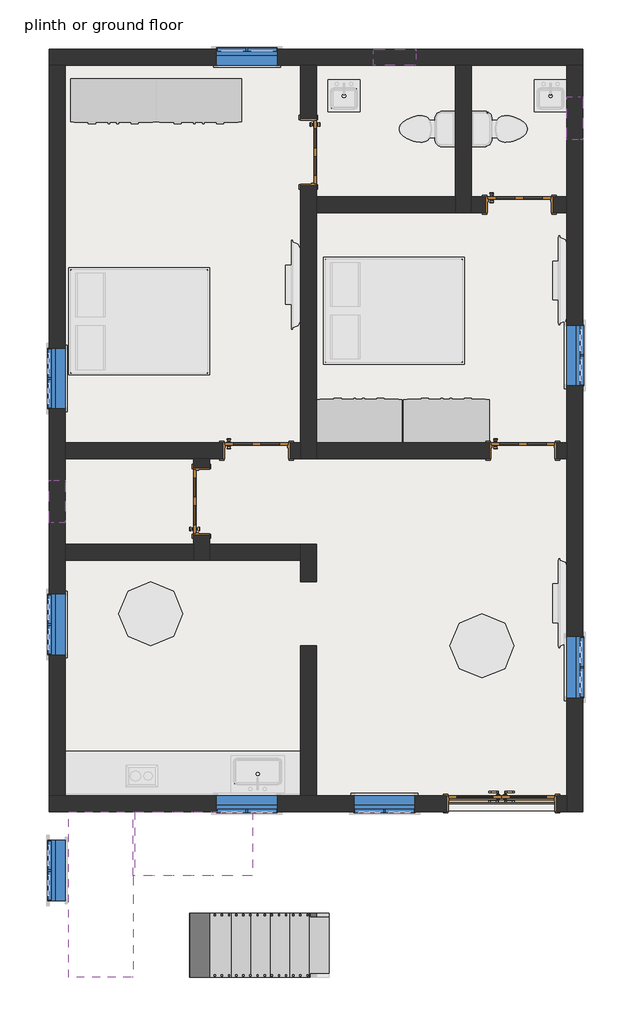
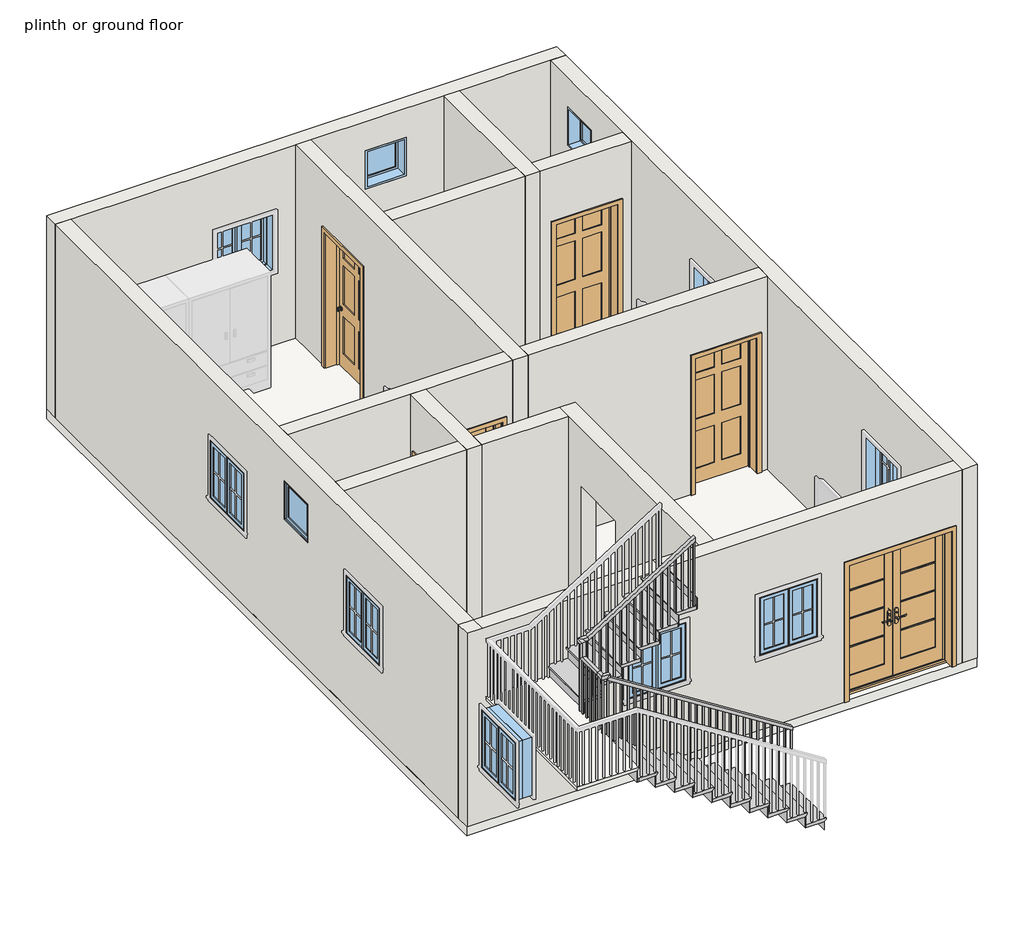
# One storey, part 1 of 3: 14 walls, 11 windows, 6 doors, 2 slabs, 2 stair flights, 1 railing.
"""IFC4 building model written with IfcOpenShell, lengths in millimetres."""

from ifc_helpers import new_model, si_unit, frame, origin, place, context, project, spatial, polyline, outline, extrude, faceted_brep, transform, mapped, element, save
from components import door_7ffae4ec, door_d86b6c54, non_monolithic_landing_b7697d37, stair_flight_c6e2231d, stair_flight_b29bf434, window_80340324, window_339605e1

model = new_model("IFC4")

# Units and contexts
model_context = context("Model", 3, world=origin())
ifc_project = project(units=[si_unit("LENGTHUNIT", "METRE", prefix="MILLI")], contexts=[model_context])

# Site, building, storey
site = spatial("IfcSite", under=ifc_project)
building = spatial("IfcBuilding", under=site)
storey = spatial("IfcBuildingStorey", under=building, Name="plinth or ground floor", Elevation=609.6)

# Doors
placement = place(None, origin())
door_shape = door_7ffae4ec(model_context)
element("IfcDoor", 1, ObjectType="Door-Exterior-Double-Full Glass-Wood_Clad : 60\" x 84\"", at=placement, inside=storey, context=model_context, shape_type="MappedRepresentation", body=[
    mapped(door_shape, transform((25464.9136801, 6450.5159313, 609.6), x_axis=(1.0, 0.0, 0.0), y_axis=(0.0, 1.0, 0.0), z_axis=(0.0, 0.0, 1.0))),
])
door_2_shape = door_d86b6c54(model_context)
element("IfcDoor", 2, ObjectType="Door-Interior-Single-6_Panel-Wood : 36\" x 84\"", at=placement, inside=storey, context=model_context, shape_type="MappedRepresentation", body=[
    mapped(door_2_shape, transform((25769.7136801, 11479.7159313, 609.6), x_axis=(1.0, 0.0, 0.0), y_axis=(0.0, 1.0, 0.0), z_axis=(0.0, 0.0, 1.0))),
])
element("IfcDoor", 3, ObjectType="Door-Interior-Single-6_Panel-Wood : 36\" x 84\"", at=placement, inside=storey, context=model_context, shape_type="MappedRepresentation", body=[
    mapped(door_2_shape, transform((21969.5484036, 11479.7159313, 609.6), x_axis=(1.0, 0.0, 0.0), y_axis=(0.0, 1.0, 0.0), z_axis=(0.0, 0.0, 1.0))),
])
element("IfcDoor", 4, ObjectType="Door-Interior-Single-6_Panel-Wood : 36\" x 84\"", at=placement, inside=storey, context=model_context, shape_type="MappedRepresentation", body=[
    mapped(door_2_shape, transform((22712.1886801, 15731.0409313, 609.6), x_axis=(0.0, -1.0, 0.0), y_axis=(1.0, 0.0, 0.0), z_axis=(0.0, 0.0, 1.0))),
])
element("IfcDoor", 5, ObjectType="Door-Interior-Single-6_Panel-Wood : 36\" x 84\"", at=placement, inside=storey, context=model_context, shape_type="MappedRepresentation", body=[
    mapped(door_2_shape, transform((25718.9136801, 14984.9159313, 609.6), x_axis=(1.0, 0.0, 0.0), y_axis=(0.0, 1.0, 0.0), z_axis=(0.0, 0.0, 1.0))),
])
element("IfcDoor", 6, ObjectType="Door-Interior-Single-6_Panel-Wood : 36\" x 84\"", at=placement, inside=storey, context=model_context, shape_type="MappedRepresentation", body=[
    mapped(door_2_shape, transform((21181.8386801, 10752.6409313, 609.6), x_axis=(0.0, 1.0, 0.0), y_axis=(-1.0, 0.0, 0.0), z_axis=(0.0, 0.0, 1.0))),
])

# Railing
element("IfcRailing", 7, ObjectType="Handrail - Rectangular", at=placement, inside=storey, context=model_context, shape_type="SolidModel", body=[
    faceted_brep([(23001.1136801, 4834.4409313, 1701.8), (23001.1136801, 4834.4409313, 1641.586276), (23001.1136801, 4885.2409313, 1641.586276), (23001.1136801, 4885.2409313, 1701.8), (20283.3136801, 4834.4409313, 3431.3090909), (20232.5136801, 4834.4409313, 3403.4226396), (20232.5136801, 4885.2409313, 3403.4226396), (20283.3136801, 4885.2409313, 3431.3090909), (20283.3136801, 4834.4409313, 3479.8), (20232.5136801, 4834.4409313, 3429.0), (20232.5136801, 4885.2409313, 3429.0), (20283.3136801, 4885.2409313, 3479.8), (20156.3136801, 4834.4409313, 3479.8), (20156.3136801, 4834.4409313, 3429.0), (20207.1136801, 4885.2409313, 3429.0), (20207.1136801, 4885.2409313, 3479.8), (20156.3136801, 4961.4409313, 3479.8), (20156.3136801, 4961.4409313, 3429.0), (20207.1136801, 4961.4409313, 3429.0), (20207.1136801, 4961.4409313, 3479.8), (20156.3136801, 5342.4409313, 3479.8), (20156.3136801, 5393.2409313, 3429.0), (20207.1136801, 5393.2409313, 3429.0), (20207.1136801, 5342.4409313, 3479.8), (20156.3136801, 5342.4409313, 3706.0909091), (20156.3136801, 5393.2409313, 3655.2909091), (20207.1136801, 5393.2409313, 3655.2909091), (20207.1136801, 5342.4409313, 3706.0909091), (20156.3136801, 5469.4409313, 3706.0909091), (20156.3136801, 5469.4409313, 3655.2909091), (20207.1136801, 5418.6409313, 3655.2909091), (20207.1136801, 5418.6409313, 3706.0909091), (20283.3136801, 5469.4409313, 3706.0909091), (20298.106675, 5469.4409313, 3655.2909091), (20298.106675, 5418.6409313, 3655.2909091), (20283.3136801, 5418.6409313, 3706.0909091), (21883.5136801, 5469.4409313, 4724.4), (21883.5136801, 5418.6409313, 4724.4), (21883.5136801, 5418.6409313, 4664.186276), (21883.5136801, 5469.4409313, 4664.186276)], [[[0, 1, 2, 3]], [[1, 0, 4, 5]], [[2, 1, 5, 6]], [[3, 2, 6, 7]], [[0, 3, 7, 4]], [[5, 4, 8, 9]], [[6, 5, 9, 10]], [[7, 6, 10, 11]], [[4, 7, 11, 8]], [[9, 8, 12, 13]], [[10, 9, 13, 14]], [[11, 10, 14, 15]], [[8, 11, 15, 12]], [[13, 12, 16, 17]], [[14, 13, 17, 18]], [[15, 14, 18, 19]], [[12, 15, 19, 16]], [[17, 16, 20, 21]], [[18, 17, 21, 22]], [[19, 18, 22, 23]], [[16, 19, 23, 20]], [[21, 20, 24, 25]], [[22, 21, 25, 26]], [[23, 22, 26, 27]], [[20, 23, 27, 24]], [[25, 24, 28, 29]], [[26, 25, 29, 30]], [[27, 26, 30, 31]], [[24, 27, 31, 28]], [[29, 28, 32, 33]], [[30, 29, 33, 34]], [[31, 30, 34, 35]], [[28, 31, 35, 32]], [[36, 37, 38, 39]], [[33, 32, 36, 39]], [[34, 33, 39, 38]], [[35, 34, 38, 37]], [[32, 35, 37, 36]]]),
    extrude(outline(polyline([(4621.7567305, 21816.8386801), (4609.6340032, 21797.7886801), (3632.2, 21797.7886801), (3632.2, 21816.8386801), (4621.7567305, 21816.8386801)])), frame((0.0, 5434.5159313, 0.0), z_axis=(0.0, 1.0, 0.0), x_axis=(0.0, 0.0, 1.0)), (0.0, 0.0, 1.0), 19.05),
    extrude(outline(polyline([(4557.1021851, 21715.2386801), (4544.9794578, 21696.1886801), (3632.2, 21696.1886801), (3632.2, 21715.2386801), (4557.1021851, 21715.2386801)])), frame((0.0, 5434.5159313, 0.0), z_axis=(0.0, 1.0, 0.0), x_axis=(0.0, 0.0, 1.0)), (0.0, 0.0, 1.0), 19.05),
    extrude(outline(polyline([(4492.4476396, 21613.6386801), (4480.3249123, 21594.5886801), (3632.2, 21594.5886801), (3632.2, 21613.6386801), (4492.4476396, 21613.6386801)])), frame((0.0, 5434.5159313, 0.0), z_axis=(0.0, 1.0, 0.0), x_axis=(0.0, 0.0, 1.0)), (0.0, 0.0, 1.0), 19.05),
    extrude(outline(polyline([(4427.7930941, 21512.0386801), (4415.6703669, 21492.9886801), (3454.4, 21492.9886801), (3454.4, 21512.0386801), (4427.7930941, 21512.0386801)])), frame((0.0, 5434.5159313, 0.0), z_axis=(0.0, 1.0, 0.0), x_axis=(0.0, 0.0, 1.0)), (0.0, 0.0, 1.0), 19.05),
    extrude(outline(polyline([(4363.1385487, 21410.4386801), (4351.0158214, 21391.3886801), (3454.4, 21391.3886801), (3454.4, 21410.4386801), (4363.1385487, 21410.4386801)])), frame((0.0, 5434.5159313, 0.0), z_axis=(0.0, 1.0, 0.0), x_axis=(0.0, 0.0, 1.0)), (0.0, 0.0, 1.0), 19.05),
    extrude(outline(polyline([(4298.4840032, 21308.8386801), (4286.361276, 21289.7886801), (3276.6, 21289.7886801), (3276.6, 21308.8386801), (4298.4840032, 21308.8386801)])), frame((0.0, 5434.5159313, 0.0), z_axis=(0.0, 1.0, 0.0), x_axis=(0.0, 0.0, 1.0)), (0.0, 0.0, 1.0), 19.05),
    extrude(outline(polyline([(4233.8294578, 21207.2386801), (4221.7067305, 21188.1886801), (3276.6, 21188.1886801), (3276.6, 21207.2386801), (4233.8294578, 21207.2386801)])), frame((0.0, 5434.5159313, 0.0), z_axis=(0.0, 1.0, 0.0), x_axis=(0.0, 0.0, 1.0)), (0.0, 0.0, 1.0), 19.05),
    extrude(outline(polyline([(4169.1749123, 21105.6386801), (4157.0521851, 21086.5886801), (3276.6, 21086.5886801), (3276.6, 21105.6386801), (4169.1749123, 21105.6386801)])), frame((0.0, 5434.5159313, 0.0), z_axis=(0.0, 1.0, 0.0), x_axis=(0.0, 0.0, 1.0)), (0.0, 0.0, 1.0), 19.05),
    extrude(outline(polyline([(4104.5203669, 21004.0386801), (4092.3976396, 20984.9886801), (3098.8, 20984.9886801), (3098.8, 21004.0386801), (4104.5203669, 21004.0386801)])), frame((0.0, 5434.5159313, 0.0), z_axis=(0.0, 1.0, 0.0), x_axis=(0.0, 0.0, 1.0)), (0.0, 0.0, 1.0), 19.05),
    extrude(outline(polyline([(4039.8658214, 20902.4386801), (4027.7430941, 20883.3886801), (3098.8, 20883.3886801), (3098.8, 20902.4386801), (4039.8658214, 20902.4386801)])), frame((0.0, 5434.5159313, 0.0), z_axis=(0.0, 1.0, 0.0), x_axis=(0.0, 0.0, 1.0)), (0.0, 0.0, 1.0), 19.05),
    extrude(outline(polyline([(3975.211276, 20800.8386801), (3963.0885487, 20781.7886801), (3098.8, 20781.7886801), (3098.8, 20800.8386801), (3975.211276, 20800.8386801)])), frame((0.0, 5434.5159313, 0.0), z_axis=(0.0, 1.0, 0.0), x_axis=(0.0, 0.0, 1.0)), (0.0, 0.0, 1.0), 19.05),
    extrude(outline(polyline([(3910.5567305, 20699.2386801), (3898.4340032, 20680.1886801), (2921.0, 20680.1886801), (2921.0, 20699.2386801), (3910.5567305, 20699.2386801)])), frame((0.0, 5434.5159313, 0.0), z_axis=(0.0, 1.0, 0.0), x_axis=(0.0, 0.0, 1.0)), (0.0, 0.0, 1.0), 19.05),
    extrude(outline(polyline([(3845.9021851, 20597.6386801), (3833.7794578, 20578.5886801), (2921.0, 20578.5886801), (2921.0, 20597.6386801), (3845.9021851, 20597.6386801)])), frame((0.0, 5434.5159313, 0.0), z_axis=(0.0, 1.0, 0.0), x_axis=(0.0, 0.0, 1.0)), (0.0, 0.0, 1.0), 19.05),
    extrude(outline(polyline([(3781.2476396, 20496.0386801), (3769.1249123, 20476.9886801), (2921.0, 20476.9886801), (2921.0, 20496.0386801), (3781.2476396, 20496.0386801)])), frame((0.0, 5434.5159313, 0.0), z_axis=(0.0, 1.0, 0.0), x_axis=(0.0, 0.0, 1.0)), (0.0, 0.0, 1.0), 19.05),
    extrude(outline(polyline([(3716.5930941, 20394.4386801), (3704.4703669, 20375.3886801), (2743.2, 20375.3886801), (2743.2, 20394.4386801), (3716.5930941, 20394.4386801)])), frame((0.0, 5434.5159313, 0.0), z_axis=(0.0, 1.0, 0.0), x_axis=(0.0, 0.0, 1.0)), (0.0, 0.0, 1.0), 19.05),
    extrude(outline(polyline([(3651.9385487, 20292.8386801), (3639.8158214, 20273.7886801), (2743.2, 20273.7886801), (2743.2, 20292.8386801), (3651.9385487, 20292.8386801)])), frame((0.0, 5434.5159313, 0.0), z_axis=(0.0, 1.0, 0.0), x_axis=(0.0, 0.0, 1.0)), (0.0, 0.0, 1.0), 19.05),
    extrude(outline(polyline([(20191.2386801, 5358.3159313), (20172.1886801, 5358.3159313), (20172.1886801, 5377.3659313), (20191.2386801, 5377.3659313), (20191.2386801, 5358.3159313)])), frame((0.0, 0.0, 2565.4), z_axis=(0.0, 0.0, 1.0), x_axis=(1.0, 0.0, 0.0)), (0.0, 0.0, 1.0), 1089.8909091),
    extrude(outline(polyline([(20191.2386801, 5256.7159313), (20172.1886801, 5256.7159313), (20172.1886801, 5275.7659313), (20191.2386801, 5275.7659313), (20191.2386801, 5256.7159313)])), frame((0.0, 0.0, 2565.4), z_axis=(0.0, 0.0, 1.0), x_axis=(1.0, 0.0, 0.0)), (0.0, 0.0, 1.0), 863.6),
    extrude(outline(polyline([(20191.2386801, 5155.1159313), (20172.1886801, 5155.1159313), (20172.1886801, 5174.1659313), (20191.2386801, 5174.1659313), (20191.2386801, 5155.1159313)])), frame((0.0, 0.0, 2565.4), z_axis=(0.0, 0.0, 1.0), x_axis=(1.0, 0.0, 0.0)), (0.0, 0.0, 1.0), 863.6),
    extrude(outline(polyline([(20191.2386801, 5053.5159313), (20172.1886801, 5053.5159313), (20172.1886801, 5072.5659313), (20191.2386801, 5072.5659313), (20191.2386801, 5053.5159313)])), frame((0.0, 0.0, 2565.4), z_axis=(0.0, 0.0, 1.0), x_axis=(1.0, 0.0, 0.0)), (0.0, 0.0, 1.0), 863.6),
    extrude(outline(polyline([(20191.2386801, 4951.9159313), (20172.1886801, 4951.9159313), (20172.1886801, 4970.9659313), (20191.2386801, 4970.9659313), (20191.2386801, 4951.9159313)])), frame((0.0, 0.0, 2565.4), z_axis=(0.0, 0.0, 1.0), x_axis=(1.0, 0.0, 0.0)), (0.0, 0.0, 1.0), 863.6),
    extrude(outline(polyline([(20267.4386801, 4869.3659313), (20267.4386801, 4850.3159313), (20248.3886801, 4850.3159313), (20248.3886801, 4869.3659313), (20267.4386801, 4869.3659313)])), frame((0.0, 0.0, 2387.6), z_axis=(0.0, 0.0, 1.0), x_axis=(1.0, 0.0, 0.0)), (0.0, 0.0, 1.0), 1041.4),
    extrude(outline(polyline([(3316.5430941, 20369.0386801), (3328.6658214, 20349.9886801), (2387.6, 20349.9886801), (2387.6, 20369.0386801), (3316.5430941, 20369.0386801)])), frame((0.0, 4850.3159313, 0.0), z_axis=(0.0, 1.0, 0.0), x_axis=(0.0, 0.0, 1.0)), (0.0, 0.0, 1.0), 19.05),
    extrude(outline(polyline([(3251.8885487, 20470.6386801), (3264.011276, 20451.5886801), (2387.6, 20451.5886801), (2387.6, 20470.6386801), (3251.8885487, 20470.6386801)])), frame((0.0, 4850.3159313, 0.0), z_axis=(0.0, 1.0, 0.0), x_axis=(0.0, 0.0, 1.0)), (0.0, 0.0, 1.0), 19.05),
    extrude(outline(polyline([(3187.2340032, 20572.2386801), (3199.3567305, 20553.1886801), (2209.8, 20553.1886801), (2209.8, 20572.2386801), (3187.2340032, 20572.2386801)])), frame((0.0, 4850.3159313, 0.0), z_axis=(0.0, 1.0, 0.0), x_axis=(0.0, 0.0, 1.0)), (0.0, 0.0, 1.0), 19.05),
    extrude(outline(polyline([(3122.5794578, 20673.8386801), (3134.7021851, 20654.7886801), (2209.8, 20654.7886801), (2209.8, 20673.8386801), (3122.5794578, 20673.8386801)])), frame((0.0, 4850.3159313, 0.0), z_axis=(0.0, 1.0, 0.0), x_axis=(0.0, 0.0, 1.0)), (0.0, 0.0, 1.0), 19.05),
    extrude(outline(polyline([(3057.9249123, 20775.4386801), (3070.0476396, 20756.3886801), (2209.8, 20756.3886801), (2209.8, 20775.4386801), (3057.9249123, 20775.4386801)])), frame((0.0, 4850.3159313, 0.0), z_axis=(0.0, 1.0, 0.0), x_axis=(0.0, 0.0, 1.0)), (0.0, 0.0, 1.0), 19.05),
    extrude(outline(polyline([(2993.2703669, 20877.0386801), (3005.3930941, 20857.9886801), (2032.0, 20857.9886801), (2032.0, 20877.0386801), (2993.2703669, 20877.0386801)])), frame((0.0, 4850.3159313, 0.0), z_axis=(0.0, 1.0, 0.0), x_axis=(0.0, 0.0, 1.0)), (0.0, 0.0, 1.0), 19.05),
    extrude(outline(polyline([(2928.6158214, 20978.6386801), (2940.7385487, 20959.5886801), (2032.0, 20959.5886801), (2032.0, 20978.6386801), (2928.6158214, 20978.6386801)])), frame((0.0, 4850.3159313, 0.0), z_axis=(0.0, 1.0, 0.0), x_axis=(0.0, 0.0, 1.0)), (0.0, 0.0, 1.0), 19.05),
    extrude(outline(polyline([(2863.961276, 21080.2386801), (2876.0840032, 21061.1886801), (1854.2, 21061.1886801), (1854.2, 21080.2386801), (2863.961276, 21080.2386801)])), frame((0.0, 4850.3159313, 0.0), z_axis=(0.0, 1.0, 0.0), x_axis=(0.0, 0.0, 1.0)), (0.0, 0.0, 1.0), 19.05),
    extrude(outline(polyline([(2799.3067305, 21181.8386801), (2811.4294578, 21162.7886801), (1854.2, 21162.7886801), (1854.2, 21181.8386801), (2799.3067305, 21181.8386801)])), frame((0.0, 4850.3159313, 0.0), z_axis=(0.0, 1.0, 0.0), x_axis=(0.0, 0.0, 1.0)), (0.0, 0.0, 1.0), 19.05),
    extrude(outline(polyline([(2734.6521851, 21283.4386801), (2746.7749123, 21264.3886801), (1854.2, 21264.3886801), (1854.2, 21283.4386801), (2734.6521851, 21283.4386801)])), frame((0.0, 4850.3159313, 0.0), z_axis=(0.0, 1.0, 0.0), x_axis=(0.0, 0.0, 1.0)), (0.0, 0.0, 1.0), 19.05),
    extrude(outline(polyline([(2669.9976396, 21385.0386801), (2682.1203669, 21365.9886801), (1676.4, 21365.9886801), (1676.4, 21385.0386801), (2669.9976396, 21385.0386801)])), frame((0.0, 4850.3159313, 0.0), z_axis=(0.0, 1.0, 0.0), x_axis=(0.0, 0.0, 1.0)), (0.0, 0.0, 1.0), 19.05),
    extrude(outline(polyline([(2605.3430941, 21486.6386801), (2617.4658214, 21467.5886801), (1676.4, 21467.5886801), (1676.4, 21486.6386801), (2605.3430941, 21486.6386801)])), frame((0.0, 4850.3159313, 0.0), z_axis=(0.0, 1.0, 0.0), x_axis=(0.0, 0.0, 1.0)), (0.0, 0.0, 1.0), 19.05),
    extrude(outline(polyline([(2540.6885487, 21588.2386801), (2552.811276, 21569.1886801), (1676.4, 21569.1886801), (1676.4, 21588.2386801), (2540.6885487, 21588.2386801)])), frame((0.0, 4850.3159313, 0.0), z_axis=(0.0, 1.0, 0.0), x_axis=(0.0, 0.0, 1.0)), (0.0, 0.0, 1.0), 19.05),
    extrude(outline(polyline([(2476.0340032, 21689.8386801), (2488.1567305, 21670.7886801), (1498.6, 21670.7886801), (1498.6, 21689.8386801), (2476.0340032, 21689.8386801)])), frame((0.0, 4850.3159313, 0.0), z_axis=(0.0, 1.0, 0.0), x_axis=(0.0, 0.0, 1.0)), (0.0, 0.0, 1.0), 19.05),
    extrude(outline(polyline([(2411.3794578, 21791.4386801), (2423.5021851, 21772.3886801), (1498.6, 21772.3886801), (1498.6, 21791.4386801), (2411.3794578, 21791.4386801)])), frame((0.0, 4850.3159313, 0.0), z_axis=(0.0, 1.0, 0.0), x_axis=(0.0, 0.0, 1.0)), (0.0, 0.0, 1.0), 19.05),
    extrude(outline(polyline([(2346.7249123, 21893.0386801), (2358.8476396, 21873.9886801), (1498.6, 21873.9886801), (1498.6, 21893.0386801), (2346.7249123, 21893.0386801)])), frame((0.0, 4850.3159313, 0.0), z_axis=(0.0, 1.0, 0.0), x_axis=(0.0, 0.0, 1.0)), (0.0, 0.0, 1.0), 19.05),
    extrude(outline(polyline([(2282.0703669, 21994.6386801), (2294.1930941, 21975.5886801), (1320.8, 21975.5886801), (1320.8, 21994.6386801), (2282.0703669, 21994.6386801)])), frame((0.0, 4850.3159313, 0.0), z_axis=(0.0, 1.0, 0.0), x_axis=(0.0, 0.0, 1.0)), (0.0, 0.0, 1.0), 19.05),
    extrude(outline(polyline([(2217.4158214, 22096.2386801), (2229.5385487, 22077.1886801), (1320.8, 22077.1886801), (1320.8, 22096.2386801), (2217.4158214, 22096.2386801)])), frame((0.0, 4850.3159313, 0.0), z_axis=(0.0, 1.0, 0.0), x_axis=(0.0, 0.0, 1.0)), (0.0, 0.0, 1.0), 19.05),
    extrude(outline(polyline([(2152.761276, 22197.8386801), (2164.8840032, 22178.7886801), (1143.0, 22178.7886801), (1143.0, 22197.8386801), (2152.761276, 22197.8386801)])), frame((0.0, 4850.3159313, 0.0), z_axis=(0.0, 1.0, 0.0), x_axis=(0.0, 0.0, 1.0)), (0.0, 0.0, 1.0), 19.05),
    extrude(outline(polyline([(2088.1067305, 22299.4386801), (2100.2294578, 22280.3886801), (1143.0, 22280.3886801), (1143.0, 22299.4386801), (2088.1067305, 22299.4386801)])), frame((0.0, 4850.3159313, 0.0), z_axis=(0.0, 1.0, 0.0), x_axis=(0.0, 0.0, 1.0)), (0.0, 0.0, 1.0), 19.05),
    extrude(outline(polyline([(2023.4521851, 22401.0386801), (2035.5749123, 22381.9886801), (1143.0, 22381.9886801), (1143.0, 22401.0386801), (2023.4521851, 22401.0386801)])), frame((0.0, 4850.3159313, 0.0), z_axis=(0.0, 1.0, 0.0), x_axis=(0.0, 0.0, 1.0)), (0.0, 0.0, 1.0), 19.05),
    extrude(outline(polyline([(1958.7976396, 22502.6386801), (1970.9203669, 22483.5886801), (965.2, 22483.5886801), (965.2, 22502.6386801), (1958.7976396, 22502.6386801)])), frame((0.0, 4850.3159313, 0.0), z_axis=(0.0, 1.0, 0.0), x_axis=(0.0, 0.0, 1.0)), (0.0, 0.0, 1.0), 19.05),
    extrude(outline(polyline([(1894.1430941, 22604.2386801), (1906.2658214, 22585.1886801), (965.2, 22585.1886801), (965.2, 22604.2386801), (1894.1430941, 22604.2386801)])), frame((0.0, 4850.3159313, 0.0), z_axis=(0.0, 1.0, 0.0), x_axis=(0.0, 0.0, 1.0)), (0.0, 0.0, 1.0), 19.05),
    extrude(outline(polyline([(1829.4885487, 22705.8386801), (1841.611276, 22686.7886801), (965.2, 22686.7886801), (965.2, 22705.8386801), (1829.4885487, 22705.8386801)])), frame((0.0, 4850.3159313, 0.0), z_axis=(0.0, 1.0, 0.0), x_axis=(0.0, 0.0, 1.0)), (0.0, 0.0, 1.0), 19.05),
    extrude(outline(polyline([(1764.8340032, 22807.4386801), (1776.9567305, 22788.3886801), (787.4, 22788.3886801), (787.4, 22807.4386801), (1764.8340032, 22807.4386801)])), frame((0.0, 4850.3159313, 0.0), z_axis=(0.0, 1.0, 0.0), x_axis=(0.0, 0.0, 1.0)), (0.0, 0.0, 1.0), 19.05),
    extrude(outline(polyline([(1700.1794578, 22909.0386801), (1712.3021851, 22889.9886801), (787.4, 22889.9886801), (787.4, 22909.0386801), (1700.1794578, 22909.0386801)])), frame((0.0, 4850.3159313, 0.0), z_axis=(0.0, 1.0, 0.0), x_axis=(0.0, 0.0, 1.0)), (0.0, 0.0, 1.0), 19.05),
    extrude(outline(polyline([(20191.2386801, 5434.5159313), (20172.1886801, 5434.5159313), (20172.1886801, 5453.5659313), (20191.2386801, 5453.5659313), (20191.2386801, 5434.5159313)])), frame((0.0, 0.0, 2565.4), z_axis=(0.0, 0.0, 1.0), x_axis=(1.0, 0.0, 0.0)), (0.0, 0.0, 1.0), 1089.8909091),
    extrude(outline(polyline([(20191.2386801, 4869.3659313), (20191.2386801, 4850.3159313), (20172.1886801, 4850.3159313), (20172.1886801, 4869.3659313), (20191.2386801, 4869.3659313)])), frame((0.0, 0.0, 2565.4), z_axis=(0.0, 0.0, 1.0), x_axis=(1.0, 0.0, 0.0)), (0.0, 0.0, 1.0), 863.6),
    extrude(outline(polyline([(4664.186276, 21883.5136801), (4652.0635487, 21864.4636801), (3632.2, 21864.4636801), (3632.2, 21883.5136801), (4664.186276, 21883.5136801)])), frame((0.0, 5434.5159313, 0.0), z_axis=(0.0, 1.0, 0.0), x_axis=(0.0, 0.0, 1.0)), (0.0, 0.0, 1.0), 19.05),
    extrude(outline(polyline([(1641.586276, 23001.1136801), (1653.7090032, 22982.0636801), (787.4, 22982.0636801), (787.4, 23001.1136801), (1641.586276, 23001.1136801)])), frame((0.0, 4850.3159313, 0.0), z_axis=(0.0, 1.0, 0.0), x_axis=(0.0, 0.0, 1.0)), (0.0, 0.0, 1.0), 19.05),
])

# Slabs
element("IfcSlab", 8, at=placement, inside=storey, context=model_context, shape_type="SweptSolid", body=[
    extrude(outline(polyline([(26620.6136801, 17196.7752787), (26620.6136801, 6349.6718948), (19013.3136801, 6349.6718948), (19013.3136801, 17196.7752787), (26620.6136801, 17196.7752787)])), frame((0.0, 0.0, 457.2), z_axis=(0.0, 0.0, 1.0), x_axis=(1.0, 0.0, 0.0)), (0.0, 0.0, 1.0), 152.4),
])
non_monolithic_landing_shape = non_monolithic_landing_b7697d37(model_context)
element("IfcSlab", 9, ObjectType="Non-Monolithic Landing", at=placement, inside=storey, context=model_context, shape_type="MappedRepresentation", body=[
    mapped(non_monolithic_landing_shape, transform((0.0, 0.0, 0.0), x_axis=(1.0, 0.0, 0.0), y_axis=(0.0, 1.0, 0.0), z_axis=(0.0, 0.0, 1.0))),
])

# Stair flights
stair_flight_shape = stair_flight_c6e2231d(model_context)
element("IfcStairFlight", 10, ObjectType="2\" Tread 1\" Nosing 1/4\" Riser", at=placement, inside=storey, context=model_context, shape_type="MappedRepresentation", body=[
    mapped(stair_flight_shape, transform((0.0, 0.0, 0.0), x_axis=(1.0, 0.0, 0.0), y_axis=(0.0, 1.0, 0.0), z_axis=(0.0, 0.0, 1.0))),
])
stair_flight_2_shape = stair_flight_b29bf434(model_context)
element("IfcStairFlight", 11, ObjectType="2\" Tread 1\" Nosing 1/4\" Riser", at=placement, inside=storey, context=model_context, shape_type="MappedRepresentation", body=[
    mapped(stair_flight_2_shape, transform((0.0, 0.0, 0.0), x_axis=(1.0, 0.0, 0.0), y_axis=(0.0, 1.0, 0.0), z_axis=(0.0, 0.0, 1.0))),
])

# Walls
element("IfcWall", 12, at=placement, inside=storey, context=model_context, shape_type="Brep", body=[
    faceted_brep([(19013.3136801, 16968.1752787, 609.6), (19241.9136801, 16968.1752787, 609.6), (22594.7136801, 16968.1752787, 609.6), (22823.3136801, 16968.1752787, 609.6), (24804.5136801, 16968.1752787, 609.6), (25033.1136801, 16968.1752787, 609.6), (26392.0136801, 16968.1752787, 609.6), (26620.6136801, 16968.1752787, 609.6), (26620.6136801, 16968.1752787, 3657.6), (26392.0136801, 16968.1752787, 3657.6), (25033.1136801, 16968.1752787, 3657.6), (24804.5136801, 16968.1752787, 3657.6), (22823.3136801, 16968.1752787, 3657.6), (22594.7136801, 16968.1752787, 3657.6), (19241.9136801, 16968.1752787, 3657.6), (19013.3136801, 16968.1752787, 3657.6), (22264.5136801, 16968.1752787, 2708.275), (22264.5136801, 16968.1752787, 1793.875), (21400.9136801, 16968.1752787, 1793.875), (21400.9136801, 16968.1752787, 2708.275), (24245.7136801, 16968.1752787, 3200.4), (24245.7136801, 16968.1752787, 2590.8), (23636.1136801, 16968.1752787, 2590.8), (23636.1136801, 16968.1752787, 3200.4), (19013.3136801, 17196.7752787, 609.6), (19013.3136801, 17196.7752787, 3657.6), (26620.6136801, 17196.7752787, 3657.6), (26620.6136801, 17196.7752787, 609.6), (22264.5136801, 17196.7752787, 2708.275), (21400.9136801, 17196.7752787, 2708.275), (21400.9136801, 17196.7752787, 1793.875), (22264.5136801, 17196.7752787, 1793.875), (24245.7136801, 17196.7752787, 3200.4), (23636.1136801, 17196.7752787, 3200.4), (23636.1136801, 17196.7752787, 2590.8), (24245.7136801, 17196.7752787, 2590.8)], [[[0, 1, 2, 3, 4, 5, 6, 7, 8, 9, 10, 11, 12, 13, 14, 15], [16, 17, 18, 19], [20, 21, 22, 23]], [[24, 25, 26, 27], [28, 29, 30, 31], [32, 33, 34, 35]], [[7, 6, 5, 4, 3, 2, 1, 0, 24, 27]], [[8, 7, 27, 26]], [[0, 15, 25, 24]], [[17, 16, 28, 31]], [[18, 17, 31, 30]], [[19, 18, 30, 29]], [[16, 19, 29, 28]], [[21, 20, 32, 35]], [[22, 21, 35, 34]], [[23, 22, 34, 33]], [[20, 23, 33, 32]], [[15, 14, 13, 12, 11, 10, 9, 8, 26, 25]]]),
])
element("IfcWall", 13, at=placement, inside=storey, context=model_context, shape_type="Brep", body=[
    faceted_brep([(26392.0136801, 16968.1752787, 609.6), (26392.0136801, 15096.0409313, 609.6), (26392.0136801, 14867.4409313, 609.6), (26392.0136801, 11590.8409313, 609.6), (26392.0136801, 11362.2409313, 609.6), (26392.0136801, 6561.6409313, 609.6), (26392.0136801, 6333.0409313, 609.6), (26392.0136801, 6333.0409313, 1066.8), (26392.0136801, 6333.0409313, 3657.6), (26392.0136801, 6561.6409313, 3657.6), (26392.0136801, 11362.2409313, 3657.6), (26392.0136801, 11590.8409313, 3657.6), (26392.0136801, 14867.4409313, 3657.6), (26392.0136801, 15096.0409313, 3657.6), (26392.0136801, 16968.1752787, 3657.6), (26392.0136801, 7958.6409313, 2708.275), (26392.0136801, 7958.6409313, 1793.875), (26392.0136801, 8822.2409313, 1793.875), (26392.0136801, 8822.2409313, 2708.275), (26392.0136801, 12403.6409313, 2708.275), (26392.0136801, 12403.6409313, 1793.875), (26392.0136801, 13267.2409313, 1793.875), (26392.0136801, 13267.2409313, 2708.275), (26392.0136801, 15908.8409313, 3200.4), (26392.0136801, 15908.8409313, 2590.8), (26392.0136801, 16518.4409313, 2590.8), (26392.0136801, 16518.4409313, 3200.4), (26620.6136801, 16968.1752787, 609.6), (26620.6136801, 16968.1752787, 3657.6), (26620.6136801, 6333.0409313, 3657.6), (26620.6136801, 6333.0409313, 1066.8), (26620.6136801, 6333.0409313, 609.6), (26620.6136801, 7958.6409313, 2708.275), (26620.6136801, 8822.2409313, 2708.275), (26620.6136801, 8822.2409313, 1793.875), (26620.6136801, 7958.6409313, 1793.875), (26620.6136801, 12403.6409313, 2708.275), (26620.6136801, 13267.2409313, 2708.275), (26620.6136801, 13267.2409313, 1793.875), (26620.6136801, 12403.6409313, 1793.875), (26620.6136801, 15908.8409313, 3200.4), (26620.6136801, 16518.4409313, 3200.4), (26620.6136801, 16518.4409313, 2590.8), (26620.6136801, 15908.8409313, 2590.8)], [[[0, 1, 2, 3, 4, 5, 6, 7, 8, 9, 10, 11, 12, 13, 14], [15, 16, 17, 18], [19, 20, 21, 22], [23, 24, 25, 26]], [[27, 28, 29, 30, 31], [32, 33, 34, 35], [36, 37, 38, 39], [40, 41, 42, 43]], [[6, 5, 4, 3, 2, 1, 0, 27, 31]], [[0, 14, 28, 27]], [[6, 31, 30, 29, 8, 7]], [[16, 15, 32, 35]], [[17, 16, 35, 34]], [[18, 17, 34, 33]], [[15, 18, 33, 32]], [[20, 19, 36, 39]], [[21, 20, 39, 38]], [[22, 21, 38, 37]], [[19, 22, 37, 36]], [[24, 23, 40, 43]], [[25, 24, 43, 42]], [[26, 25, 42, 41]], [[23, 26, 41, 40]], [[14, 13, 12, 11, 10, 9, 8, 29, 28]]]),
])
element("IfcWall", 14, at=placement, inside=storey, context=model_context, shape_type="Brep", body=[
    faceted_brep([(22594.7136801, 16968.1752787, 3657.6), (22594.7136801, 16968.1752787, 609.6), (22594.7136801, 16213.6409313, 609.6), (22594.7136801, 16213.6409313, 2768.6), (22594.7136801, 15248.4409313, 2768.6), (22594.7136801, 15248.4409313, 609.6), (22594.7136801, 11590.8409313, 609.6), (22594.7136801, 11362.2409313, 609.6), (22594.7136801, 11362.2409313, 3657.6), (22594.7136801, 11590.8409313, 3657.6), (22823.3136801, 16968.1752787, 609.6), (22823.3136801, 16968.1752787, 3657.6), (22823.3136801, 15096.0409313, 3657.6), (22823.3136801, 14867.4409313, 3657.6), (22823.3136801, 11590.8409313, 3657.6), (22823.3136801, 11362.2409313, 3657.6), (22823.3136801, 11362.2409313, 609.6), (22823.3136801, 11590.8409313, 609.6), (22823.3136801, 14867.4409313, 609.6), (22823.3136801, 15096.0409313, 609.6), (22823.3136801, 15248.4409313, 609.6), (22823.3136801, 15248.4409313, 2768.6), (22823.3136801, 16213.6409313, 2768.6), (22823.3136801, 16213.6409313, 609.6)], [[[0, 1, 2, 3, 4, 5, 6, 7, 8, 9]], [[10, 11, 12, 13, 14, 15, 16, 17, 18, 19, 20, 21, 22, 23]], [[1, 10, 23, 2]], [[16, 7, 6, 5, 20, 19, 18, 17]], [[1, 0, 11, 10]], [[8, 7, 16, 15]], [[4, 21, 20, 5]], [[21, 4, 3, 22]], [[22, 3, 2, 23]], [[0, 9, 8, 15, 14, 13, 12, 11]]]),
])
element("IfcWall", 15, at=placement, inside=storey, context=model_context, shape_type="Brep", body=[
    faceted_brep([(22594.7136801, 11590.8409313, 3657.6), (22594.7136801, 11590.8409313, 609.6), (22452.1484036, 11590.8409313, 609.6), (22452.1484036, 11590.8409313, 2768.6), (21486.9484036, 11590.8409313, 2768.6), (21486.9484036, 11590.8409313, 609.6), (19241.9136801, 11590.8409313, 609.6), (19241.9136801, 11590.8409313, 3657.6), (22594.7136801, 11362.2409313, 609.6), (22594.7136801, 11362.2409313, 3657.6), (21299.3136801, 11362.2409313, 3657.6), (21070.7136801, 11362.2409313, 3657.6), (19241.9136801, 11362.2409313, 3657.6), (19241.9136801, 11362.2409313, 609.6), (21070.7136801, 11362.2409313, 609.6), (21299.3136801, 11362.2409313, 609.6), (21486.9484036, 11362.2409313, 609.6), (21486.9484036, 11362.2409313, 2768.6), (22452.1484036, 11362.2409313, 2768.6), (22452.1484036, 11362.2409313, 609.6)], [[[0, 1, 2, 3, 4, 5, 6, 7]], [[8, 9, 10, 11, 12, 13, 14, 15, 16, 17, 18, 19]], [[1, 8, 19, 2]], [[13, 6, 5, 16, 15, 14]], [[1, 0, 9, 8]], [[7, 6, 13, 12]], [[18, 3, 2, 19]], [[3, 18, 17, 4]], [[4, 17, 16, 5]], [[0, 7, 12, 11, 10, 9]]]),
])
element("IfcWall", 16, at=placement, inside=storey, context=model_context, shape_type="Brep", body=[
    faceted_brep([(24804.5136801, 16968.1752787, 609.6), (24804.5136801, 15096.0409313, 609.6), (24804.5136801, 14867.4409313, 609.6), (24804.5136801, 14867.4409313, 3657.6), (24804.5136801, 15096.0409313, 3657.6), (24804.5136801, 16968.1752787, 3657.6), (25033.1136801, 16968.1752787, 609.6), (25033.1136801, 16968.1752787, 3657.6), (25033.1136801, 15096.0409313, 3657.6), (25033.1136801, 14867.4409313, 3657.6), (25033.1136801, 14867.4409313, 609.6), (25033.1136801, 15096.0409313, 609.6)], [[[0, 1, 2, 3, 4, 5]], [[6, 7, 8, 9, 10, 11]], [[2, 1, 0, 6, 11, 10]], [[0, 5, 7, 6]], [[3, 2, 10, 9]], [[5, 4, 3, 9, 8, 7]]]),
])
element("IfcWall", 17, at=placement, inside=storey, context=model_context, shape_type="SweptSolid", body=[
    extrude(outline(polyline([(22823.3136801, 15096.0409313), (24804.5136801, 15096.0409313), (24804.5136801, 14867.4409313), (22823.3136801, 14867.4409313), (22823.3136801, 15096.0409313)])), frame((0.0, 0.0, 609.6), z_axis=(0.0, 0.0, 1.0), x_axis=(1.0, 0.0, 0.0)), (0.0, 0.0, 1.0), 3048.0),
])
element("IfcWall", 18, at=placement, inside=storey, context=model_context, shape_type="SweptSolid", body=[
    extrude(outline(polyline([(3657.6, 25033.1136801), (609.6, 25033.1136801), (609.6, 25236.3136801), (2768.6, 25236.3136801), (2768.6, 26201.5136801), (609.6, 26201.5136801), (609.6, 26392.0136801), (3657.6, 26392.0136801), (3657.6, 25033.1136801)])), frame((0.0, 14867.4409313, 0.0), z_axis=(0.0, 1.0, 0.0), x_axis=(0.0, 0.0, 1.0)), (0.0, 0.0, 1.0), 228.6),
])
element("IfcWall", 19, at=placement, inside=storey, context=model_context, shape_type="SweptSolid", body=[
    extrude(outline(polyline([(3657.6, 22823.3136801), (609.6, 22823.3136801), (609.6, 25287.1136801), (2768.6, 25287.1136801), (2768.6, 26252.3136801), (609.6, 26252.3136801), (609.6, 26392.0136801), (3657.6, 26392.0136801), (3657.6, 22823.3136801)])), frame((0.0, 11362.2409313, 0.0), z_axis=(0.0, 1.0, 0.0), x_axis=(0.0, 0.0, 1.0)), (0.0, 0.0, 1.0), 228.6),
])
element("IfcWall", 20, at=placement, inside=storey, context=model_context, shape_type="Brep", body=[
    faceted_brep([(21070.7136801, 11362.2409313, 3657.6), (21070.7136801, 11362.2409313, 609.6), (21070.7136801, 11235.2409313, 609.6), (21070.7136801, 11235.2409313, 2768.6), (21070.7136801, 10270.0409313, 2768.6), (21070.7136801, 10270.0409313, 609.6), (21070.7136801, 10143.0409313, 609.6), (21070.7136801, 9914.4409313, 609.6), (21070.7136801, 9914.4409313, 3657.6), (21070.7136801, 10143.0409313, 3657.6), (21299.3136801, 11362.2409313, 609.6), (21299.3136801, 11362.2409313, 3657.6), (21299.3136801, 10143.0409313, 3657.6), (21299.3136801, 9914.4409313, 3657.6), (21299.3136801, 9914.4409313, 609.6), (21299.3136801, 10143.0409313, 609.6), (21299.3136801, 10270.0409313, 609.6), (21299.3136801, 10270.0409313, 2768.6), (21299.3136801, 11235.2409313, 2768.6), (21299.3136801, 11235.2409313, 609.6)], [[[0, 1, 2, 3, 4, 5, 6, 7, 8, 9]], [[10, 11, 12, 13, 14, 15, 16, 17, 18, 19]], [[1, 10, 19, 2]], [[14, 7, 6, 5, 16, 15]], [[1, 0, 11, 10]], [[8, 7, 14, 13]], [[18, 3, 2, 19]], [[3, 18, 17, 4]], [[4, 17, 16, 5]], [[0, 9, 8, 13, 12, 11]]]),
])
element("IfcWall", 21, at=placement, inside=storey, context=model_context, shape_type="SweptSolid", body=[
    extrude(outline(polyline([(19241.9136801, 10143.0409313), (21070.7136801, 10143.0409313), (21070.7136801, 9914.4409313), (19241.9136801, 9914.4409313), (19241.9136801, 10143.0409313)])), frame((0.0, 0.0, 609.6), z_axis=(0.0, 0.0, 1.0), x_axis=(1.0, 0.0, 0.0)), (0.0, 0.0, 1.0), 3048.0),
])
element("IfcWall", 22, at=placement, inside=storey, context=model_context, shape_type="Brep", body=[
    faceted_brep([(22594.7136801, 10143.0409313, 3657.6), (22594.7136801, 10143.0409313, 609.6), (22594.7136801, 9914.4409313, 609.6), (22594.7136801, 9609.6409313, 609.6), (22594.7136801, 9609.6409313, 2743.2), (22594.7136801, 8695.2409313, 2743.2), (22594.7136801, 8695.2409313, 609.6), (22594.7136801, 6561.6409313, 609.6), (22594.7136801, 6561.6409313, 3657.6), (22594.7136801, 9914.4409313, 3657.6), (22823.3136801, 10143.0409313, 609.6), (22823.3136801, 10143.0409313, 3657.6), (22823.3136801, 6561.6409313, 3657.6), (22823.3136801, 6561.6409313, 609.6), (22823.3136801, 8695.2409313, 609.6), (22823.3136801, 8695.2409313, 2743.2), (22823.3136801, 9609.6409313, 2743.2), (22823.3136801, 9609.6409313, 609.6)], [[[0, 1, 2, 3, 4, 5, 6, 7, 8, 9]], [[10, 11, 12, 13, 14, 15, 16, 17]], [[1, 10, 17, 3, 2]], [[13, 7, 6, 14]], [[1, 0, 11, 10]], [[8, 7, 13, 12]], [[16, 4, 3, 17]], [[5, 15, 14, 6]], [[4, 16, 15, 5]], [[0, 9, 8, 12, 11]]]),
])
element("IfcWall", 23, at=placement, inside=storey, context=model_context, shape_type="SweptSolid", body=[
    extrude(outline(polyline([(22594.7136801, 9914.4409313), (21299.3136801, 9914.4409313), (21299.3136801, 10143.0409313), (22594.7136801, 10143.0409313), (22594.7136801, 9914.4409313)])), frame((0.0, 0.0, 609.6), z_axis=(0.0, 0.0, 1.0), x_axis=(1.0, 0.0, 0.0)), (0.0, 0.0, 1.0), 3048.0),
])
element("IfcWall", 24, at=placement, inside=storey, context=model_context, shape_type="Brep", body=[
    faceted_brep([(26392.0136801, 6333.0409313, 609.6), (26392.0136801, 6333.0409313, 3657.6), (21908.9136801, 6333.0409313, 3657.6), (19241.9136801, 6333.0409313, 3657.6), (19013.3136801, 6333.0409313, 3657.6), (19013.3136801, 6333.0409313, 609.6), (24677.5136801, 6333.0409313, 609.6), (24677.5136801, 6333.0409313, 2768.6), (26252.3136801, 6333.0409313, 2768.6), (26252.3136801, 6333.0409313, 609.6), (23363.0636801, 6333.0409313, 2708.275), (24226.6636801, 6333.0409313, 2708.275), (24226.6636801, 6333.0409313, 1793.875), (23363.0636801, 6333.0409313, 1793.875), (21400.9136801, 6333.0409313, 2708.275), (22264.5136801, 6333.0409313, 2708.275), (22264.5136801, 6333.0409313, 1793.875), (21400.9136801, 6333.0409313, 1793.875), (26392.0136801, 6561.6409313, 3657.6), (26392.0136801, 6561.6409313, 609.6), (26252.3136801, 6561.6409313, 609.6), (26252.3136801, 6561.6409313, 2768.6), (24677.5136801, 6561.6409313, 2768.6), (24677.5136801, 6561.6409313, 609.6), (22823.3136801, 6561.6409313, 609.6), (22594.7136801, 6561.6409313, 609.6), (19241.9136801, 6561.6409313, 609.6), (19013.3136801, 6561.6409313, 609.6), (19013.3136801, 6561.6409313, 3657.6), (19241.9136801, 6561.6409313, 3657.6), (21908.9136801, 6561.6409313, 3657.6), (22594.7136801, 6561.6409313, 3657.6), (22823.3136801, 6561.6409313, 3657.6), (23363.0636801, 6561.6409313, 2708.275), (23363.0636801, 6561.6409313, 1793.875), (24226.6636801, 6561.6409313, 1793.875), (24226.6636801, 6561.6409313, 2708.275), (21400.9136801, 6561.6409313, 2708.275), (21400.9136801, 6561.6409313, 1793.875), (22264.5136801, 6561.6409313, 1793.875), (22264.5136801, 6561.6409313, 2708.275)], [[[0, 1, 2, 3, 4, 5, 6, 7, 8, 9], [10, 11, 12, 13], [14, 15, 16, 17]], [[18, 19, 20, 21, 22, 23, 24, 25, 26, 27, 28, 29, 30, 31, 32], [33, 34, 35, 36], [37, 38, 39, 40]], [[19, 0, 9, 20]], [[5, 27, 26, 25, 24, 23, 6]], [[0, 19, 18, 1]], [[5, 4, 28, 27]], [[8, 21, 20, 9]], [[21, 8, 7, 22]], [[22, 7, 6, 23]], [[34, 33, 10, 13]], [[35, 34, 13, 12]], [[36, 35, 12, 11]], [[33, 36, 11, 10]], [[38, 37, 14, 17]], [[39, 38, 17, 16]], [[40, 39, 16, 15]], [[37, 40, 15, 14]], [[30, 29, 3, 2]], [[2, 1, 18, 32, 31, 30]], [[4, 3, 29, 28]]]),
])
element("IfcWall", 25, at=placement, inside=storey, context=model_context, shape_type="Brep", body=[
    faceted_brep([(19241.9136801, 6561.6409313, 609.6), (19241.9136801, 9914.4409313, 609.6), (19241.9136801, 10143.0409313, 609.6), (19241.9136801, 11362.2409313, 609.6), (19241.9136801, 11590.8409313, 609.6), (19241.9136801, 16968.1752787, 609.6), (19241.9136801, 16968.1752787, 3657.6), (19241.9136801, 11590.8409313, 3657.6), (19241.9136801, 11362.2409313, 3657.6), (19241.9136801, 10143.0409313, 3657.6), (19241.9136801, 9914.4409313, 3657.6), (19241.9136801, 6724.5096261, 3657.6), (19241.9136801, 6561.6409313, 3657.6), (19241.9136801, 12937.0409313, 2708.275), (19241.9136801, 12937.0409313, 1793.875), (19241.9136801, 12073.4409313, 1793.875), (19241.9136801, 12073.4409313, 2708.275), (19241.9136801, 9431.8409313, 2708.275), (19241.9136801, 9431.8409313, 1793.875), (19241.9136801, 8568.2409313, 1793.875), (19241.9136801, 8568.2409313, 2708.275), (19241.9136801, 11057.4409313, 3200.4), (19241.9136801, 11057.4409313, 2590.8), (19241.9136801, 10447.8409313, 2590.8), (19241.9136801, 10447.8409313, 3200.4), (19013.3136801, 6561.6409313, 609.6), (19013.3136801, 6561.6409313, 3657.6), (19013.3136801, 16968.1752787, 3657.6), (19013.3136801, 16968.1752787, 609.6), (19013.3136801, 12937.0409313, 2708.275), (19013.3136801, 12073.4409313, 2708.275), (19013.3136801, 12073.4409313, 1793.875), (19013.3136801, 12937.0409313, 1793.875), (19013.3136801, 9431.8409313, 2708.275), (19013.3136801, 8568.2409313, 2708.275), (19013.3136801, 8568.2409313, 1793.875), (19013.3136801, 9431.8409313, 1793.875), (19013.3136801, 11057.4409313, 3200.4), (19013.3136801, 10447.8409313, 3200.4), (19013.3136801, 10447.8409313, 2590.8), (19013.3136801, 11057.4409313, 2590.8)], [[[0, 1, 2, 3, 4, 5, 6, 7, 8, 9, 10, 11, 12], [13, 14, 15, 16], [17, 18, 19, 20], [21, 22, 23, 24]], [[25, 26, 27, 28], [29, 30, 31, 32], [33, 34, 35, 36], [37, 38, 39, 40]], [[5, 4, 3, 2, 1, 0, 25, 28]], [[6, 5, 28, 27]], [[0, 12, 26, 25]], [[14, 13, 29, 32]], [[15, 14, 32, 31]], [[16, 15, 31, 30]], [[13, 16, 30, 29]], [[18, 17, 33, 36]], [[19, 18, 36, 35]], [[20, 19, 35, 34]], [[17, 20, 34, 33]], [[22, 21, 37, 40]], [[23, 22, 40, 39]], [[24, 23, 39, 38]], [[21, 24, 38, 37]], [[12, 11, 10, 9, 8, 7, 6, 27, 26]]]),
])

# Windows
window_shape = window_80340324(model_context)
element("IfcWindow", 26, ObjectType="Fixed : 24\" x 24\"", at=placement, inside=storey, context=model_context, shape_type="MappedRepresentation", body=[
    mapped(window_shape, transform((23979.0136801, 17082.4752787, 1676.4), x_axis=(1.0, 0.0, 0.0), y_axis=(0.0, 1.0, 0.0), z_axis=(0.0, 0.0, 1.0))),
])
element("IfcWindow", 27, ObjectType="Fixed : 24\" x 24\"", at=placement, inside=storey, context=model_context, shape_type="MappedRepresentation", body=[
    mapped(window_shape, transform((26506.3136801, 16175.5409313, 1676.4), x_axis=(0.0, -1.0, 0.0), y_axis=(1.0, 0.0, 0.0), z_axis=(0.0, 0.0, 1.0))),
])
element("IfcWindow", 28, ObjectType="Fixed : 24\" x 24\"", at=placement, inside=storey, context=model_context, shape_type="MappedRepresentation", body=[
    mapped(window_shape, transform((19127.6136801, 10790.7409313, 1676.4), x_axis=(0.0, 1.0, 0.0), y_axis=(-1.0, 0.0, 0.0), z_axis=(0.0, 0.0, 1.0))),
])
window_2_shape = window_339605e1(model_context)
element("IfcWindow", 29, ObjectType="Window-Casement-Double : 34\" x 36\"", at=placement, inside=storey, context=model_context, shape_type="MappedRepresentation", body=[
    mapped(window_2_shape, transform((23794.8636801, 6447.3409313, 879.475), x_axis=(-1.0, 0.0, 0.0), y_axis=(0.0, -1.0, 0.0), z_axis=(0.0, 0.0, 1.0))),
])
element("IfcWindow", 30, ObjectType="Window-Casement-Double : 34\" x 36\"", at=placement, inside=storey, context=model_context, shape_type="MappedRepresentation", body=[
    mapped(window_2_shape, transform((26506.3136801, 8390.4409313, 879.475), x_axis=(0.0, -1.0, 0.0), y_axis=(1.0, 0.0, 0.0), z_axis=(0.0, 0.0, 1.0))),
])
element("IfcWindow", 31, ObjectType="Window-Casement-Double : 34\" x 36\"", at=placement, inside=storey, context=model_context, shape_type="MappedRepresentation", body=[
    mapped(window_2_shape, transform((26506.3136801, 12835.4409313, 879.475), x_axis=(0.0, -1.0, 0.0), y_axis=(1.0, 0.0, 0.0), z_axis=(0.0, 0.0, 1.0))),
])
element("IfcWindow", 32, ObjectType="Window-Casement-Double : 34\" x 36\"", at=placement, inside=storey, context=model_context, shape_type="MappedRepresentation", body=[
    mapped(window_2_shape, transform((21832.7136801, 17082.4752787, 879.475), x_axis=(1.0, 0.0, 0.0), y_axis=(0.0, 1.0, 0.0), z_axis=(0.0, 0.0, 1.0))),
])
element("IfcWindow", 33, ObjectType="Window-Casement-Double : 34\" x 36\"", at=placement, inside=storey, context=model_context, shape_type="MappedRepresentation", body=[
    mapped(window_2_shape, transform((19127.6136801, 12505.2409313, 879.475), x_axis=(0.0, 1.0, 0.0), y_axis=(-1.0, 0.0, 0.0), z_axis=(0.0, 0.0, 1.0))),
])
element("IfcWindow", 34, ObjectType="Window-Casement-Double : 34\" x 36\"", at=placement, inside=storey, context=model_context, shape_type="MappedRepresentation", body=[
    mapped(window_2_shape, transform((19127.6136801, 9000.0409313, 879.475), x_axis=(0.0, 1.0, 0.0), y_axis=(-1.0, 0.0, 0.0), z_axis=(0.0, 0.0, 1.0))),
])
element("IfcWindow", 35, ObjectType="Window-Casement-Double : 34\" x 36\"", at=placement, inside=storey, context=model_context, shape_type="MappedRepresentation", body=[
    mapped(window_2_shape, transform((21832.7136801, 6447.3409313, 879.475), x_axis=(-1.0, 0.0, 0.0), y_axis=(0.0, -1.0, 0.0), z_axis=(0.0, 0.0, 1.0))),
])
element("IfcWindow", 36, ObjectType="Window-Casement-Double : 34\" x 36\"", at=placement, inside=storey, context=model_context, shape_type="MappedRepresentation", body=[
    mapped(window_2_shape, transform((19127.6136801, 5494.8409313, 879.475), x_axis=(0.0, 1.0, 0.0), y_axis=(-1.0, 0.0, 0.0), z_axis=(0.0, 0.0, 1.0))),
])

save(model, "model.ifc")

# Revit data of these elements
# Type "Door-Exterior-Double-Full Glass-Wood_Clad : 60\" x 84\""
#   Type Mark = "8"
#   Assembly Code = "B2030100"
#   Analytic Construction = "French door, wood frame with double glass"
#   Top Rail = 0' - 4 11/16"
#   Threshold Offset [instance default] = 0' - 0 1/2"
#   Thickness = 0' - 1 3/8"
#   Thermal Resistance (R) = 1.9158 (h·ft²·°F)/BTU
#   Swing Angle [instance default] = 90.00°
#   Stiles = 0' - 4 3/4"
#   Rough Width = 5' - 2"
#   Rough Height = 7' - 1"
#   Panel Width = 2' - 6"
#   Door Offset [instance default] = 0' - 0"
#   Height = 7' - 0"
#   Width = 5' - 0"
#   Heat Transfer Coefficient (U) = 0.5220 BTU/(h·ft²·°F)
#   Bottom Rail = 0' - 9 1/8"
#   Exterior Trim [instance default] = yes
#   Threshold [instance default] = yes
#   Show Grill [instance default] = yes
#   Function = 1
#   Trim Material = Cherry
#   Threshold Material = Cherry
#   Panel Material = Cherry
#   Glazing = Glass
#   Frame Material = Cherry
#   Door Handle Material = Aluminum
#   Visual Light Transmittance = 0
#   Solar Heat Gain Coefficient = 0
#   Wall Closure = (empty or 0)
#   Construction Type = (empty or 0)
# Type "Door-Interior-Single-6_Panel-Wood : 36\" x 84\""
#   Type Mark = "9"
#   Assembly Code = "C1020300"
#   Analytic Construction = "Wooden"
#   Top Rail = 0' - 4 11/16"
#   Top Panel = 0' - 11"
#   Thickness = 0' - 1 3/8"
#   Thermal Resistance (R) = 2.5876 (h·ft²·°F)/BTU
#   Swing Angle [instance default] = 90.00°
#   Stiles = 0' - 4 3/4"
#   Rough Width = 3' - 2"
#   Rough Height = 7' - 1"
#   Mullion = 0' - 4 1/2"
#   Lock Rail = 0' - 7 1/2"
#   Intermediate Rail = 0' - 4 1/2"
#   Height = 7' - 0"
#   Width = 3' - 0"
#   Heat Transfer Coefficient (U) = 0.3865 BTU/(h·ft²·°F)
#   Bottom Rail = 0' - 9 1/8"
#   Trim Material = Cherry
#   Panel Material = Cherry
#   Frame Material = Cherry
#   Door Handle Material = Aluminum
#   Visual Light Transmittance = 0
#   Solar Heat Gain Coefficient = 0
#   Wall Closure = (empty or 0)
#   Function = (empty or 0)
# Type "Handrail - Rectangular"
#   Assembly Code = "C2010400"
#   built-in parameter 1008612 = 0.0416667 (stored number, unit not read)
#   built-in parameter 1008611 = 0.0416667 (stored number, unit not read)
#   built-in parameter 1008609 = 0.333333 (stored number, unit not read)
#   built-in parameter 1008604 = 0.166667 (stored number, unit not read)
#   built-in parameter 1008603 = 0.166667 (stored number, unit not read)
#   Railing Height = 3' - 0"
#   built-in parameter 1008630 = 2
#   built-in parameter 1008610 = 2
#   built-in parameter 1008618 = Baluster - Square : 3/4"
# Type
#   Assembly Code = "B1010"
#   Function = 0
#   Layers, outside or top first: 0' - 6" "Concrete, Cast-in-Place gray" (function 1)
# Type
#   Assembly Code = "B2010"
#   Layers, outside or top first: 0' - 9" no material (function 1)
# Type "Fixed : 24\" x 24\""
#   Type Mark = "3"
#   Construction Type Id = "GSP4R"
#   Assembly Code = "B2020100"
#   Analytic Construction = "1/8 in Pilkington single glazing"
#   Visual Light Transmittance = 0.9
#   Solar Heat Gain Coefficient = 0.78
#   Heat Transfer Coefficient (U) = 0.6496 BTU/(h·ft²·°F)
#   Height = 2' - 0"
#   Default Sill Height = 3' - 0"
#   Width = 2' - 0"
#   Window Inset = 0' - 0 3/4"
#   Define Thermal Properties by = 1
#   Define Thermal Properties by = 1
#   Glass Pane Material = Glass
#   Sash Material = Sash
#   Wall Closure = (empty or 0)
# Type "Window-Casement-Double : 34\" x 36\""
#   Type Mark = "14"
#   Fire Rating = "0.5h"
#   Assembly Code = "B2020100"
#   Analytic Construction = "Double glazing - domestic"
#   Frame Extension [instance default] = 0' - 0 1/4"
#   Window Inset [instance default] = 0' - 0"
#   Wall Thickness [instance default] = 0' - 6"
#   Interior Wall Closure [instance default] = 0' - 2 1/4"
#   Half Width = 1' - 5"
#   Visual Light Transmittance = 0.81
#   Thermal Resistance (R) = 1.8146 (h·ft²·°F)/BTU
#   Solar Heat Gain Coefficient = 0.76
#   Rough Width = 2' - 10 1/2"
#   Rough Height = 3' - 0 1/2"
#   Height = 3' - 0"
#   Heat Transfer Coefficient (U) = 0.5511 BTU/(h·ft²·°F)
#   Exterior Wall Closure [instance default] = 0' - 1 1/4"
#   Extension Jamb [instance default] = 0' - 2 1/4"
#   Default Sill Height = 3' - 0"
#   Width = 2' - 10"
#   Define Thermal Properties by = 0
#   Muntin Visibility = yes
#   Interior Trim Visibility [instance default] = yes
#   Exterior Trim Visibility [instance default] = yes
#   Extension Jamb Visibility [instance default] = yes
#   Interior Trim Material = Wood - Stained
#   Muntin Pattern = Muntin Pattern_2x2 : Muntin Pattern_2x2
#   Interior Trim = Trim-Window-Interior-Flat : Picture Frame
#   Interior Frame Material = Wood - Stained
#   Glass Panel Material = Glass
#   Exterior Trim Material = Clad - White
#   Exterior Trim = Trim-Window-Exterior-Flat : with Sill
#   Exterior Frame Material = Clad - White
#   Wall Closure = (empty or 0)
# Element 1 (IfcDoor, "Door-Exterior-Double-Full Glass-Wood_Clad : 60\" x 84\"")
#   Threshold Offset = 0' - 0 1/2"
#   Swing Angle = 90.00°
#   Door Offset = 0' - 0"
#   Threshold = yes
#   Show Grill = yes
#   Exterior Trim = yes
#   Phase Created = New Construction
#   Materials on its faces: "Cherry", "Aluminum", "Glass"
# Elements 2, 3, 4, 5, 6 (IfcDoor, "Door-Interior-Single-6_Panel-Wood : 36\" x 84\"")
#   Swing Angle = 90.00°
#   Phase Created = New Construction
#   Materials on its faces: "Cherry", "Aluminum"
# Element 7 (IfcRailing, "Handrail - Rectangular")
#   Phase Created = New Construction
# Element 8 (IfcSlab)
#   Height Offset From Level = 0' - 0"
#   Phase Created = New Construction
#   Materials on its faces: "Concrete, Cast-in-Place gray", "Laminate, Ivory, Matte"
# Element 9 (IfcSlab, "Non-Monolithic Landing")
#   Phase Created = New Construction
# Elements 10, 11 (IfcStairFlight, "2\" Tread 1\" Nosing 1/4\" Riser")
#   Phase Created = New Construction
# Element 12 (IfcWall)
#   Top Offset = 0' - 0"
#   Base Offset = 0' - 0"
#   wall height = 10' - 0"
#   Phase Created = New Construction
#   Base Constraint = plinth or ground floor
#   Top Constraint = 1st floor
#   Materials on its faces: "Default Wall", "Birch"
# Element 13 (IfcWall)
#   Top Offset = 0' - 0"
#   Base Offset = 0' - 0"
#   wall height = 10' - 0"
#   Phase Created = New Construction
#   Base Constraint = plinth or ground floor
#   Top Constraint = 1st floor
#   Materials on its faces: "Default Wall", "Birch", "Laminate, Ivory, Matte"
# Elements 14, 15, 16, 17, 18, 19, 20, 21, 22, 23, 24, 25 (IfcWall)
#   Top Offset = 0' - 0"
#   Base Offset = 0' - 0"
#   wall height = 10' - 0"
#   Phase Created = New Construction
#   Base Constraint = plinth or ground floor
#   Top Constraint = 1st floor
#   Materials on its faces: "Default Wall"
# Element 26 (IfcWindow, "Fixed : 24\" x 24\"")
#   Mark = "8"
#   Phase Created = New Construction
#   Materials on its faces: "Sash", "Glass"
# Element 27 (IfcWindow, "Fixed : 24\" x 24\"")
#   Mark = "9"
#   Phase Created = New Construction
#   Materials on its faces: "Sash", "Glass"
# Element 28 (IfcWindow, "Fixed : 24\" x 24\"")
#   Mark = "10"
#   Phase Created = New Construction
#   Materials on its faces: "Sash", "Glass"
# Element 29 (IfcWindow, "Window-Casement-Double : 34\" x 36\"")
#   Mark = "1"
#   Window Inset = 0' - 0"
#   Interior Wall Closure = 0' - 2 1/4"
#   Frame Extension = 0' - 0 1/4"
#   Exterior Wall Closure = 0' - 1 1/4"
#   Interior Trim Visibility = yes
#   Exterior Trim Visibility = yes
#   Phase Created = New Construction
#   Materials on its faces: "Wood - Stained", "Glass", "Clad - White"
# Element 30 (IfcWindow, "Window-Casement-Double : 34\" x 36\"")
#   Mark = "2"
#   Window Inset = 0' - 0"
#   Interior Wall Closure = 0' - 2 1/4"
#   Frame Extension = 0' - 0 1/4"
#   Exterior Wall Closure = 0' - 1 1/4"
#   Interior Trim Visibility = yes
#   Exterior Trim Visibility = yes
#   Phase Created = New Construction
#   Materials on its faces: "Wood - Stained", "Glass", "Clad - White"
# Element 31 (IfcWindow, "Window-Casement-Double : 34\" x 36\"")
#   Mark = "3"
#   Window Inset = 0' - 0"
#   Interior Wall Closure = 0' - 2 1/4"
#   Frame Extension = 0' - 0 1/4"
#   Exterior Wall Closure = 0' - 1 1/4"
#   Interior Trim Visibility = yes
#   Exterior Trim Visibility = yes
#   Phase Created = New Construction
#   Materials on its faces: "Wood - Stained", "Glass", "Clad - White"
# Element 32 (IfcWindow, "Window-Casement-Double : 34\" x 36\"")
#   Mark = "4"
#   Window Inset = 0' - 0"
#   Interior Wall Closure = 0' - 2 1/4"
#   Frame Extension = 0' - 0 1/4"
#   Exterior Wall Closure = 0' - 1 1/4"
#   Interior Trim Visibility = yes
#   Exterior Trim Visibility = yes
#   Phase Created = New Construction
#   Materials on its faces: "Wood - Stained", "Glass", "Clad - White"
# Element 33 (IfcWindow, "Window-Casement-Double : 34\" x 36\"")
#   Mark = "5"
#   Window Inset = 0' - 0"
#   Interior Wall Closure = 0' - 2 1/4"
#   Frame Extension = 0' - 0 1/4"
#   Exterior Wall Closure = 0' - 1 1/4"
#   Interior Trim Visibility = yes
#   Exterior Trim Visibility = yes
#   Phase Created = New Construction
#   Materials on its faces: "Wood - Stained", "Glass", "Clad - White"
# Element 34 (IfcWindow, "Window-Casement-Double : 34\" x 36\"")
#   Mark = "6"
#   Window Inset = 0' - 0"
#   Interior Wall Closure = 0' - 2 1/4"
#   Frame Extension = 0' - 0 1/4"
#   Exterior Wall Closure = 0' - 1 1/4"
#   Interior Trim Visibility = yes
#   Exterior Trim Visibility = yes
#   Phase Created = New Construction
#   Materials on its faces: "Wood - Stained", "Glass", "Clad - White"
# Element 35 (IfcWindow, "Window-Casement-Double : 34\" x 36\"")
#   Mark = "7"
#   Window Inset = 0' - 0"
#   Interior Wall Closure = 0' - 2 1/4"
#   Frame Extension = 0' - 0 1/4"
#   Exterior Wall Closure = 0' - 1 1/4"
#   Interior Trim Visibility = yes
#   Exterior Trim Visibility = yes
#   Phase Created = New Construction
#   Materials on its faces: "Wood - Stained", "Glass", "Clad - White"
